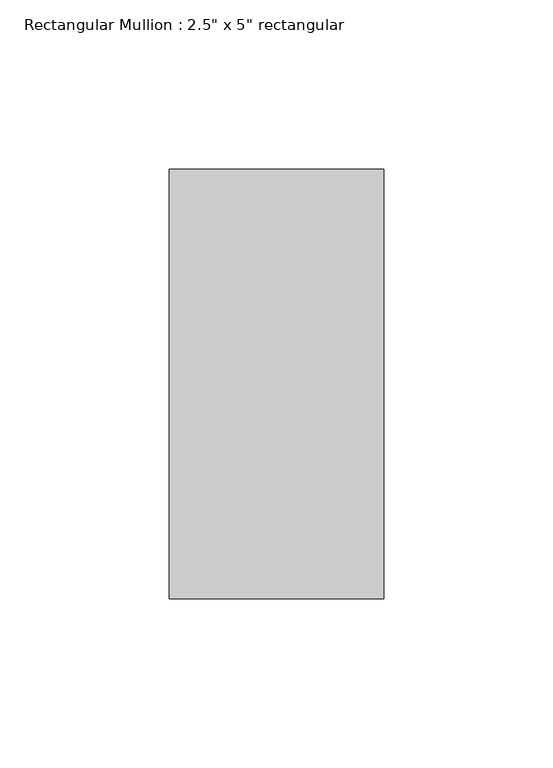
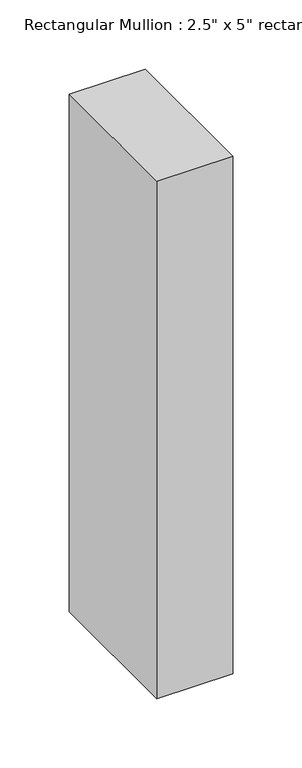
"""IFC4 building model written with IfcOpenShell, lengths in millimetres: member geometry."""

from ifc_helpers import new_model, si_unit, frame, origin, place, context, project, spatial, polyline, outline, extrude, source, transform, mapped, element, save


def member_ffd4c858(model_context):
    return source(origin(), model_context, "Body", "SweptSolid", [
        extrude(outline(polyline([(31.75, 63.5), (31.75, -63.5), (-31.75, -63.5), (-31.75, 63.5), (31.75, 63.5)])), frame((0.0, 0.0, -457.2), z_axis=(0.0, 0.0, 1.0), x_axis=(1.0, 0.0, 0.0)), (0.0, 0.0, 1.0), 457.2),
    ])


if __name__ == "__main__":
    model = new_model("IFC4")
    model_context = context("Model", 3, world=origin())
    ifc_project = project(units=[si_unit("LENGTHUNIT", "METRE", prefix="MILLI")], contexts=[model_context])
    site = spatial("IfcSite", under=ifc_project)
    building = spatial("IfcBuilding", under=site)
    placement = place(None, origin())
    member_shape = member_ffd4c858(model_context)
    element("IfcMember", 1, ObjectType="Rectangular Mullion : 2.5\" x 5\" rectangular", at=placement, inside=building, context=model_context, shape_type="MappedRepresentation", body=[
        mapped(member_shape, transform((0.0, 0.0, 0.0), x_axis=(1.0, 0.0, 0.0), y_axis=(0.0, 1.0, 0.0), z_axis=(0.0, 0.0, 1.0))),
    ])
    save(model, "model.ifc")

# Revit data of these elements
# Type "Rectangular Mullion : 2.5\" x 5\" rectangular"
#   built-in parameter 1007304 = 0.416667 (stored number, unit not read)
#   built-in parameter 1007301 = 0.104167 (stored number, unit not read)
#   built-in parameter 1007300 = 0.104167 (stored number, unit not read)
# Element 1 (IfcMember, "Rectangular Mullion : 2.5\" x 5\" rectangular")
#   Materials on its faces: "Aluminum"
# Materials
#   "Aluminum": class "Metal", colour RGB 247 247 247, transparency 0, Description = "Aluminum 6061", Cost = 0
